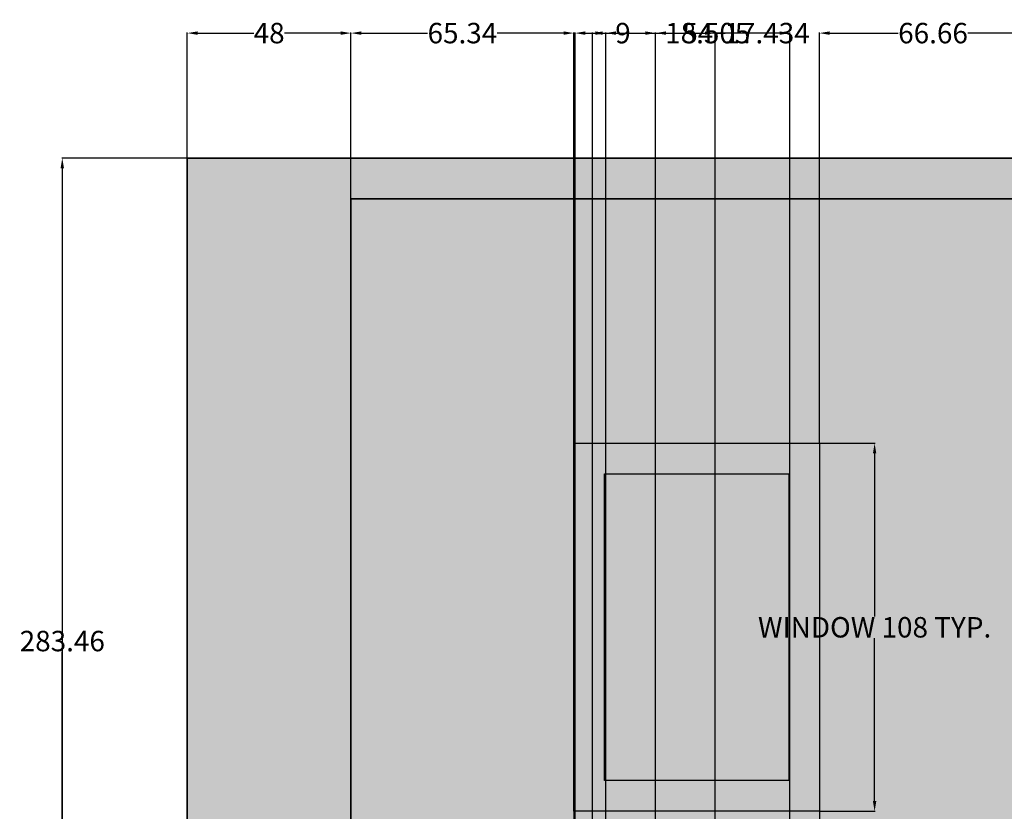
# Model space of a CAD drawing. Units: inches. Extents: x 126 to 726, y 86 to 888.
# Tile 8 of 13: x 137 to 426, y 655 to 888. Entities that reach past the tile are written whole.
import ezdxf

# ---------------------------------------------------------------- set-up
doc = ezdxf.new("R2010")
doc.units = ezdxf.units.IN
doc.header["$MEASUREMENT"] = 0
for name, color, linetype, lineweight in [('A-ANNO-DIMS', 2, 'Continuous', 18), ('A-ELEV', 7, 'Continuous', 35), ('A-ELEV-PATT', 8, 'Continuous', 13), ('A-GLAZ', 4, 'Continuous', 25)]:
    doc.layers.add(name, color=color, linetype=linetype, lineweight=lineweight)
doc.styles.get("Standard").update_dxf_attribs({"font": 'arial.ttf'})
doc.dimstyles.get("Standard").update_dxf_attribs({"dimtxt": 6, "dimasz": 3, "dimexe": 0.18, "dimexo": 0.0625, "dimgap": 0.09, "dimtad": 0, "dimtih": 1, "dimtoh": 1, "dimdec": 0, "dimzin": 0, "dimdsep": 46, "dimlunit": 3, "dimtxsty": 'Standard', "dimcen": 0.09, "dimadec": 0, "dimazin": 0, "dimtfac": 1, "dimtdec": 0, "dimtofl": 0, "dimtmove": 0, "dimatfit": 3, "dimfxl": 1, "dimtolj": 1, "dimtzin": 0, "dimarcsym": 0})

# ---------------------------------------------------------------- blocks, each defined once
blk = doc.blocks.new('WIN-FRAME')
for points in [[(72, 0), (0, 0), (0, 108), (72, 108)], [(63, 9), (9, 9), (9, 99), (63, 99)]]:
    blk.add_lwpolyline(points, close=True)
blk = doc.blocks.new('*D5')
at = {"layer": 'A-ANNO-DIMS', "color": 0, "lineweight": -2, "transparency": 16777216}
for p, q in [((371.38, 763.35), (387.7, 763.35)), ((387.52, 760.35), (387.52, 712.55)), ((387.52, 658.35), (387.52, 706.16)), ((371.38, 655.35), (387.7, 655.35))]:
    blk.add_line(p, q, dxfattribs=at)
at = {"layer": 'A-ANNO-DIMS', "color": 0, "transparency": 16777216}
for points in [[(387.02, 760.35), (388.02, 760.35), (387.52, 763.35)], [(387.02, 658.35), (388.02, 658.35), (387.52, 655.35)]]:
    blk.add_solid(points, dxfattribs=at)
at = {"layer": 'Defpoints', "color": 0, "transparency": 16777216}
for p in [(371.32, 763.35), (387.52, 763.35), (371.32, 655.35)]:
    blk.add_point(p, dxfattribs=at)
at = {"layer": 'A-ANNO-DIMS', "color": 0, "transparency": 16777216, "insert": (387.52, 709.35), "char_height": 6, "attachment_point": 5}
blk.add_mtext('\\A1;WINDOW 108 TYP.', dxfattribs=at)
blk = doc.blocks.new('*D6')
at = {"layer": 'A-ANNO-DIMS', "color": 0, "lineweight": -2, "transparency": 16777216}
for p, q in [((299.32, 655.29), (299.32, 638.97)), ((371.32, 655.29), (371.32, 638.97)), ((302.32, 639.15), (320.65, 639.15)), ((368.32, 639.15), (349.99, 639.15))]:
    blk.add_line(p, q, dxfattribs=at)
at = {"layer": 'A-ANNO-DIMS', "color": 0, "transparency": 16777216}
for points in [[(302.32, 639.65), (302.32, 638.65), (299.32, 639.15)], [(368.32, 639.65), (368.32, 638.65), (371.32, 639.15)]]:
    blk.add_solid(points, dxfattribs=at)
at = {"layer": 'Defpoints', "color": 0, "transparency": 16777216}
for p in [(299.32, 655.35), (371.32, 655.35), (371.32, 639.15)]:
    blk.add_point(p, dxfattribs=at)
at = {"layer": 'A-ANNO-DIMS', "color": 0, "transparency": 16777216, "insert": (335.32, 639.15), "char_height": 6, "attachment_point": 5}
blk.add_mtext('\\A1;72 TYP.', dxfattribs=at)
blk = doc.blocks.new('*D14')
at = {"layer": 'A-ANNO-DIMS', "color": 0, "lineweight": -2, "transparency": 16777216}
for p, q in [((185.91, 847.04), (149.14, 847.04)), ((149.32, 844.04), (149.32, 490.2)), ((149.32, 130.04), (149.32, 483.89)), ((185.91, 127.04), (149.14, 127.04))]:
    blk.add_line(p, q, dxfattribs=at)
at = {"layer": 'A-ANNO-DIMS', "color": 0, "transparency": 16777216}
for points in [[(148.82, 844.04), (149.82, 844.04), (149.32, 847.04)], [(148.82, 130.04), (149.82, 130.04), (149.32, 127.04)]]:
    blk.add_solid(points, dxfattribs=at)
at = {"layer": 'Defpoints', "color": 0, "transparency": 16777216}
for p in [(149.32, 847.04), (185.97, 847.04), (185.97, 127.04)]:
    blk.add_point(p, dxfattribs=at)
at = {"layer": 'A-ANNO-DIMS', "color": 0, "transparency": 16777216, "insert": (149.32, 487.04), "char_height": 6, "attachment_point": 5}
blk.add_mtext('\\A1;720', dxfattribs=at)
blk = doc.blocks.new('*D22')
at = {"layer": 'A-ANNO-DIMS', "color": 0, "lineweight": -2, "transparency": 16777216}
for p, q in [((185.91, 847.04), (149.14, 847.04)), ((149.32, 844.04), (149.32, 708.47)), ((149.32, 566.58), (149.32, 702.16)), ((431.28, 563.58), (149.14, 563.58))]:
    blk.add_line(p, q, dxfattribs=at)
at = {"layer": 'A-ANNO-DIMS', "color": 0, "transparency": 16777216}
for points in [[(148.82, 844.04), (149.82, 844.04), (149.32, 847.04)], [(148.82, 566.58), (149.82, 566.58), (149.32, 563.58)]]:
    blk.add_solid(points, dxfattribs=at)
at = {"layer": 'Defpoints', "color": 0, "transparency": 16777216}
for p in [(149.32, 847.04), (185.97, 847.04), (431.34, 563.58)]:
    blk.add_point(p, dxfattribs=at)
at = {"layer": 'A-ANNO-DIMS', "color": 0, "transparency": 16777216, "insert": (149.32, 705.31), "char_height": 6, "attachment_point": 5}
blk.add_mtext('\\A1;283.46', dxfattribs=at)
blk = doc.blocks.new('*D23')
at = {"layer": 'A-ANNO-DIMS', "color": 0, "lineweight": -2, "transparency": 16777216}
for p, q in [((185.97, 847.1), (185.97, 883.87)), ((188.97, 883.69), (205.46, 883.69)), ((230.97, 883.69), (214.49, 883.69)), ((233.97, 835.1), (233.97, 883.87))]:
    blk.add_line(p, q, dxfattribs=at)
at = {"layer": 'A-ANNO-DIMS', "color": 0, "transparency": 16777216}
for points in [[(188.97, 884.19), (188.97, 883.19), (185.97, 883.69)], [(230.97, 884.19), (230.97, 883.19), (233.97, 883.69)]]:
    blk.add_solid(points, dxfattribs=at)
at = {"layer": 'Defpoints', "color": 0, "transparency": 16777216}
for p in [(233.97, 883.69), (185.97, 847.04), (233.97, 835.04)]:
    blk.add_point(p, dxfattribs=at)
at = {"layer": 'A-ANNO-DIMS', "color": 0, "transparency": 16777216, "insert": (209.97, 883.69), "char_height": 6, "attachment_point": 5}
blk.add_mtext('\\A1;48', dxfattribs=at)
blk = doc.blocks.new('*D24')
at = {"layer": 'A-ANNO-DIMS', "color": 0, "lineweight": -2, "transparency": 16777216}
for p, q in [((233.97, 835.1), (233.97, 883.87)), ((236.97, 883.69), (256.43, 883.69)), ((296.32, 883.69), (276.86, 883.69)), ((299.32, 763.42), (299.32, 883.87))]:
    blk.add_line(p, q, dxfattribs=at)
at = {"layer": 'A-ANNO-DIMS', "color": 0, "transparency": 16777216}
for points in [[(236.97, 884.19), (236.97, 883.19), (233.97, 883.69)], [(296.32, 884.19), (296.32, 883.19), (299.32, 883.69)]]:
    blk.add_solid(points, dxfattribs=at)
at = {"layer": 'Defpoints', "color": 0, "transparency": 16777216}
for p in [(299.32, 883.69), (233.97, 835.04), (299.32, 763.35)]:
    blk.add_point(p, dxfattribs=at)
at = {"layer": 'A-ANNO-DIMS', "color": 0, "transparency": 16777216, "insert": (266.65, 883.69), "char_height": 6, "attachment_point": 5}
blk.add_mtext('\\A1;65.34', dxfattribs=at)
blk = doc.blocks.new('*D25')
at = {"layer": 'A-ANNO-DIMS', "color": 0, "lineweight": -2, "transparency": 16777216}
for p, q in [((371.32, 763.42), (371.32, 883.87)), ((374.32, 883.69), (394.42, 883.69)), ((434.97, 883.69), (414.87, 883.69)), ((437.97, 826.04), (437.97, 883.87))]:
    blk.add_line(p, q, dxfattribs=at)
at = {"layer": 'A-ANNO-DIMS', "color": 0, "transparency": 16777216}
for points in [[(374.32, 884.19), (374.32, 883.19), (371.32, 883.69)], [(434.97, 884.19), (434.97, 883.19), (437.97, 883.69)]]:
    blk.add_solid(points, dxfattribs=at)
at = {"layer": 'Defpoints', "color": 0, "transparency": 16777216}
for p in [(437.97, 883.69), (437.97, 825.98), (371.32, 763.35)]:
    blk.add_point(p, dxfattribs=at)
at = {"layer": 'A-ANNO-DIMS', "color": 0, "transparency": 16777216, "insert": (404.65, 883.69), "char_height": 6, "attachment_point": 5}
blk.add_mtext('\\A1;66.66', dxfattribs=at)
blk = doc.blocks.new('*D32')
at = {"layer": 'A-ANNO-DIMS', "color": 0, "lineweight": -2, "transparency": 16777216}
for p, q in [((299.67, 533.75), (299.67, 883.87)), ((302.67, 883.69), (305.67, 883.69)), ((308.67, 524.75), (308.67, 883.87)), ((308.67, 883.69), (311.67, 883.69))]:
    blk.add_line(p, q, dxfattribs=at)
at = {"layer": 'A-ANNO-DIMS', "color": 0, "transparency": 16777216}
for points in [[(302.67, 884.19), (302.67, 883.19), (299.67, 883.69)], [(305.67, 884.19), (305.67, 883.19), (308.67, 883.69)]]:
    blk.add_solid(points, dxfattribs=at)
at = {"layer": 'Defpoints', "color": 0, "transparency": 16777216}
for p in [(308.67, 883.69), (299.67, 533.68), (308.67, 524.68)]:
    blk.add_point(p, dxfattribs=at)
at = {"layer": 'A-ANNO-DIMS', "color": 0, "transparency": 16777216, "insert": (313.73, 883.69), "char_height": 6, "attachment_point": 5}
blk.add_mtext('\\A1;9', dxfattribs=at)
blk = doc.blocks.new('*D33')
at = {"layer": 'A-ANNO-DIMS', "color": 0, "lineweight": -2, "transparency": 16777216}
for p, q in [((308.67, 524.75), (308.67, 883.87)), ((311.67, 883.69), (331.29, 883.69)), ((359.67, 883.69), (340.04, 883.69)), ((362.67, 524.75), (362.67, 883.87))]:
    blk.add_line(p, q, dxfattribs=at)
at = {"layer": 'A-ANNO-DIMS', "color": 0, "transparency": 16777216}
for points in [[(311.67, 884.19), (311.67, 883.19), (308.67, 883.69)], [(359.67, 884.19), (359.67, 883.19), (362.67, 883.69)]]:
    blk.add_solid(points, dxfattribs=at)
at = {"layer": 'Defpoints', "color": 0, "transparency": 16777216}
for p in [(362.67, 883.69), (308.67, 524.68), (362.67, 524.68)]:
    blk.add_point(p, dxfattribs=at)
at = {"layer": 'A-ANNO-DIMS', "color": 0, "transparency": 16777216, "insert": (335.67, 883.69), "char_height": 6, "attachment_point": 5}
blk.add_mtext('\\A1;54', dxfattribs=at)
blk = doc.blocks.new('*D38')
at = {"layer": 'A-ANNO-DIMS', "color": 0, "lineweight": -2, "transparency": 16777216}
for p, q in [((304.8, 168.3), (304.8, 883.87)), ((307.8, 883.69), (320.3, 883.69)), ((323.3, 174.45), (323.3, 883.87)), ((323.3, 883.69), (326.3, 883.69))]:
    blk.add_line(p, q, dxfattribs=at)
at = {"layer": 'A-ANNO-DIMS', "color": 0, "transparency": 16777216}
for points in [[(307.8, 884.19), (307.8, 883.19), (304.8, 883.69)], [(320.3, 884.19), (320.3, 883.19), (323.3, 883.69)]]:
    blk.add_solid(points, dxfattribs=at)
at = {"layer": 'Defpoints', "color": 0, "transparency": 16777216}
for p in [(323.3, 883.69), (323.3, 174.39), (304.8, 168.24)]:
    blk.add_point(p, dxfattribs=at)
at = {"layer": 'A-ANNO-DIMS', "color": 0, "transparency": 16777216, "insert": (338.59, 883.69), "char_height": 6, "attachment_point": 5}
blk.add_mtext('\\A1;18.505', dxfattribs=at)
blk = doc.blocks.new('*D39')
at = {"layer": 'A-ANNO-DIMS', "color": 0, "lineweight": -2, "transparency": 16777216}
for p, q in [((323.3, 174.45), (323.3, 883.87)), ((326.3, 883.69), (337.74, 883.69)), ((340.74, 168.3), (340.74, 883.87)), ((340.74, 883.69), (343.74, 883.69))]:
    blk.add_line(p, q, dxfattribs=at)
at = {"layer": 'A-ANNO-DIMS', "color": 0, "transparency": 16777216}
for points in [[(326.3, 884.19), (326.3, 883.19), (323.3, 883.69)], [(337.74, 884.19), (337.74, 883.19), (340.74, 883.69)]]:
    blk.add_solid(points, dxfattribs=at)
at = {"layer": 'Defpoints', "color": 0, "transparency": 16777216}
for p in [(340.74, 883.69), (323.3, 174.39), (340.74, 168.24)]:
    blk.add_point(p, dxfattribs=at)
at = {"layer": 'A-ANNO-DIMS', "color": 0, "transparency": 16777216, "insert": (355.99, 883.69), "char_height": 6, "attachment_point": 5}
blk.add_mtext('\\A1;17.434', dxfattribs=at)

msp = doc.modelspace()

# ---------------------------------------------------------------- hatches: boundary and pattern name
at = {"layer": 'A-ELEV-PATT'}
h = msp.add_hatch(color=256, dxfattribs=at)
h.dxf.hatch_style = 1
h.paths.add_polyline_path([(233.9749, 545.5846), (431.3386, 545.5846), (431.3386, 563.5846), (185.9749, 563.5846), (185.9749, 395.5846), (431.3386, 395.5846), (431.3386, 413.5846), (233.9749, 413.5846)])
h.paths.add_polyline_path([(233.9749, 835.0424), (485.9749, 835.0424), (605.9749, 835.0424), (605.9749, 847.0424), (485.9749, 847.0424), (185.9749, 847.0424), (185.9749, 606.5846), (233.9749, 606.5846)])
h.paths.add_polyline_path([(233.9749, 597.5846), (185.9749, 597.5846), (185.9749, 585.5846), (233.9749, 585.5846)])
h.paths.add_polyline_path([(233.9749, 580.5846), (185.9749, 580.5846), (185.9749, 568.5846), (233.9749, 568.5846)])
h = msp.add_hatch(color=256, dxfattribs=at)
h.dxf.hatch_style = 1
h.paths.add_polyline_path([(437.9749, 499.1312), (485.9749, 499.1312), (485.9749, 501.4423), (437.9749, 501.4423), (437.9749, 513.4423), (485.9749, 513.4423), (485.9749, 515.7534), (437.9749, 515.7534), (437.9749, 527.7534), (485.9749, 527.7534), (485.9749, 530.0646), (437.9749, 530.0646), (437.9749, 542.0646), (485.9749, 542.0646), (485.9749, 544.3757), (437.9749, 544.3757), (437.9749, 556.3757), (485.9749, 556.3757), (485.9749, 558.6868), (437.9749, 558.6868), (437.9749, 570.6868), (485.9749, 570.6868), (485.9749, 572.9979), (437.9749, 572.9979), (437.9749, 584.9979), (485.9749, 584.9979), (485.9749, 587.309), (437.9749, 587.309), (437.9749, 595.0424), (429.9749, 595.0424), (429.9749, 607.0424), (437.9749, 607.0424), (437.9749, 615.9312), (437.9749, 630.2423), (437.9749, 642.2423), (485.9749, 642.2423), (485.9749, 644.5534), (437.9749, 644.5534), (437.9749, 656.5534), (485.9749, 656.5534), (485.9749, 658.8645), (437.9749, 658.8645), (437.9749, 670.8645), (485.9749, 670.8645), (485.9749, 673.1757), (437.9749, 673.1757), (437.9749, 685.1757), (485.9749, 685.1757), (485.9749, 687.4868), (437.9749, 687.4868), (437.9749, 699.4868), (485.9749, 699.4868), (485.9749, 701.7979), (437.9749, 701.7979), (437.9749, 713.7979), (485.9749, 713.7979), (485.9749, 716.109), (437.9749, 716.109), (437.9749, 728.109), (485.9749, 728.109), (485.9749, 730.4201), (437.9749, 730.4201), (437.9749, 742.4201), (485.9749, 742.4201), (485.9749, 744.7312), (437.9749, 744.7312), (437.9749, 756.7312), (485.9749, 756.7312), (485.9749, 759.0423), (437.9749, 759.0423), (437.9749, 771.0423), (485.9749, 771.0423), (485.9749, 773.3534), (437.9749, 773.3534), (437.9749, 785.3534), (485.9749, 785.3534), (485.9749, 787.6645), (437.9749, 787.6645), (437.9749, 799.6645), (485.9749, 799.6645), (485.9749, 801.9756), (437.9749, 801.9756), (437.9749, 811.2868), (485.9749, 811.2868), (485.9749, 813.9756), (437.9749, 813.9756), (437.9749, 825.9756), (485.9749, 825.9756), (485.9749, 835.0424), (233.9749, 835.0424), (233.9749, 606.5846), (185.9749, 606.5846), (185.9749, 597.5846), (233.9749, 597.5846), (233.9749, 585.5846), (185.9749, 585.5846), (185.9749, 580.5846), (233.9749, 580.5846), (233.9749, 568.5846), (185.9749, 568.5846), (185.9749, 563.5846), (431.3386, 563.5846), (431.3386, 545.5846), (233.9749, 545.5846), (233.9749, 413.5846), (431.3386, 413.5846), (431.3386, 395.5846), (185.9749, 395.5846), (185.9749, 386.5846), (233.9749, 386.5846), (233.9749, 374.5846), (185.9749, 374.5846), (185.9749, 369.5846), (233.9749, 369.5846), (233.9749, 357.5846), (185.9749, 357.5846), (185.9749, 352.5846), (233.9749, 352.5846), (233.9749, 340.5846), (185.9749, 340.5846), (185.9749, 331.5846), (233.9749, 331.5846), (233.9749, 127.0424), (485.9749, 127.0424), (485.9749, 129.3535), (437.9749, 129.3535), (437.9749, 141.3535), (485.9749, 141.3535), (485.9749, 143.6646), (437.9749, 143.6646), (437.9749, 155.6646), (485.9749, 155.6646), (485.9749, 157.9757), (437.9749, 157.9757), (437.9749, 169.9757), (485.9749, 169.9757), (485.9749, 172.2868), (437.9749, 172.2868), (437.9749, 184.2868), (485.9749, 184.2868), (485.9749, 186.5979), (437.9749, 186.5979), (437.9749, 198.5979), (485.9749, 198.5979), (485.9749, 200.909), (437.9749, 200.909), (437.9749, 212.909), (485.9749, 212.909), (485.9749, 215.2201), (437.9749, 215.2201), (437.9749, 227.2201), (485.9749, 227.2201), (485.9749, 229.5312), (437.9749, 229.5312), (437.9749, 241.5312), (485.9749, 241.5312), (485.9749, 243.8424), (437.9749, 243.8424), (437.9749, 255.8424), (485.9749, 255.8424), (485.9749, 258.1535), (437.9749, 258.1535), (437.9749, 270.1535), (485.9749, 270.1535), (485.9749, 272.4646), (437.9749, 272.4646), (437.9749, 284.4646), (485.9749, 284.4646), (485.9749, 286.7757), (437.9749, 286.7757), (437.9749, 298.7757), (485.9749, 298.7757), (485.9749, 301.0868), (437.9749, 301.0868), (437.9749, 313.0868), (485.9749, 313.0868), (485.9749, 315.3979), (437.9749, 315.3979), (437.9749, 327.3979), (485.9749, 327.3979), (485.9749, 329.709), (437.9749, 329.709), (437.9749, 341.709), (485.9749, 341.709), (485.9749, 344.0201), (437.9749, 344.0201), (437.9749, 355.0424), (429.9749, 355.0424), (429.9749, 367.0424), (437.9749, 367.0424), (437.9749, 372.6423), (437.9749, 386.9535), (437.9749, 401.2646), (437.9749, 413.2646), (485.9749, 413.2646), (485.9749, 415.5757), (437.9749, 415.5757), (437.9749, 427.5757), (485.9749, 427.5757), (485.9749, 429.8868), (437.9749, 429.8868), (437.9749, 441.8868), (485.9749, 441.8868), (485.9749, 444.1979), (437.9749, 444.1979), (437.9749, 456.1979), (485.9749, 456.1979), (485.9749, 458.509), (437.9749, 458.509), (437.9749, 470.509), (485.9749, 470.509), (485.9749, 472.8201), (437.9749, 472.8201), (437.9749, 484.8201), (485.9749, 484.8201), (485.9749, 487.1312), (437.9749, 487.1312)])
h.paths.add_polyline_path([(299.6658, 533.6845), (371.6658, 533.6845), (371.6658, 425.6845), (299.6658, 425.6845)], flags=16)
h.paths.add_polyline_path([(308.6658, 524.6845), (362.6658, 524.6845), (362.6658, 434.6845), (308.6658, 434.6845)], flags=0)
h.paths.add_polyline_path([(317.7956, 603.3211, -0.4129833), (306.8418, 614.321, -0.94403766), (328.769, 615.5845, -0.04423165), (330.7031, 615.4048, -0.89973713), (352.5798, 615.6161, -0.4129833), (363.5336, 604.6162, -0.94403766), (341.6064, 603.3528, -0.04423165), (339.6723, 603.5324, -0.89973713)], flags=16)
h.paths.add_polyline_path([(319.7228, 604.5846, -0.02633223), (319.7726, 605.5306, -0.47905713), (308.8418, 614.321, -1), (326.8418, 614.321, -0.02633223), (326.7919, 613.375, -0.17413188), (332.826, 612.5948, -0.04918553), (332.6526, 614.3527, -1), (350.6526, 614.3527, -0.02633223), (350.6028, 613.4067, -0.47905713), (361.5336, 604.6162, -1), (343.5336, 604.6162, -0.02633223), (343.5834, 605.5622, -0.17413188), (337.5494, 606.3424, -0.04918553), (337.7228, 604.5846, -1)], flags=0)
h.paths.add_polyline_path([(328.769, 355.6561, -0.04423165), (330.7031, 355.4765, -0.89973713), (352.5798, 355.6878, -0.4129833), (363.5336, 344.6879, -0.94403766), (341.6064, 343.4244, -0.04423165), (339.6723, 343.604, -0.89973713), (317.7956, 343.3927, -0.4129833), (306.8418, 354.3926, -0.94403766)], flags=16)
h.paths.add_polyline_path([(326.8418, 354.3926, -0.02633223), (326.7919, 353.4466, -0.17413188), (332.826, 352.6664, -0.04918553), (332.6526, 354.4243, -1), (350.6526, 354.4243, -0.02633223), (350.6028, 353.4783, -0.47905713), (361.5336, 344.6879, -1), (343.5336, 344.6879, -0.02633223), (343.5834, 345.6339, -0.17413188), (337.5494, 346.4141, -0.04918553), (337.7228, 344.6562, -1), (319.7228, 344.6562, -0.02633223), (319.7726, 345.6022, -0.47905713), (308.8418, 354.3926, -1)], flags=0)
h.paths.add_polyline_path([(299.3189, 655.3527), (299.3189, 763.3527), (371.3189, 763.3527), (371.3189, 655.3527)], flags=16)
h.paths.add_polyline_path([(308.3189, 664.3527), (308.3189, 754.3527), (362.3189, 754.3527), (362.3189, 664.3527)], flags=0)
h.paths.add_polyline_path([(299.6658, 303.5875), (371.6658, 303.5875), (371.6658, 195.5875), (299.6658, 195.5875)], flags=16)
h.paths.add_polyline_path([(308.6658, 294.5875), (362.6658, 294.5875), (362.6658, 204.5875), (308.6658, 204.5875)], flags=0)
h.paths.add_polyline_path([(326.3038, 177.3867), (346.055, 177.3867, -0.41421356), (349.055, 174.3867), (349.055, 171.2378), (363.489, 171.2378, -0.41421356), (366.489, 168.2378), (366.489, 159.7133, -0.41421356), (363.489, 156.7133), (343.7379, 156.7133, -0.41421356), (340.7379, 159.7133), (340.7379, 162.8622), (330.5504, 162.8622), (330.5504, 159.7133, -0.41421356), (327.5504, 156.7133), (307.7992, 156.7133, -0.41421356), (304.7992, 159.7133), (304.7992, 168.2378, -0.41421356), (307.7992, 171.2378), (323.3038, 171.2378), (323.3038, 174.3867, -0.41421356)], flags=16)
h.paths.add_polyline_path([(326.3038, 175.3867), (346.055, 175.3867, -0.41421356), (347.055, 174.3867), (347.055, 169.2378), (363.489, 169.2378, -0.41421356), (364.489, 168.2378), (364.489, 159.7133, -0.41421356), (363.489, 158.7133), (343.7379, 158.7133, -0.41421356), (342.7379, 159.7133), (342.7379, 164.8622), (328.5504, 164.8622), (328.5504, 159.7133, -0.41421356), (327.5504, 158.7133), (307.7992, 158.7133, -0.41421356), (306.7992, 159.7133), (306.7992, 168.2378, -0.41421356), (307.7992, 169.2378), (325.3038, 169.2378), (325.3038, 174.3867, -0.41421356)], flags=0)
h = msp.add_hatch(dxfattribs=at)
h.set_pattern_fill('GRAVEL', color=256, scale=40)
h.paths.add_polyline_path([(437.9749, 642.2423), (485.9749, 642.2423), (485.9749, 644.5534), (437.9749, 644.5534), (437.9749, 656.5534), (485.9749, 656.5534), (485.9749, 658.8645), (437.9749, 658.8645), (437.9749, 670.8645), (485.9749, 670.8645), (485.9749, 673.1757), (437.9749, 673.1757), (437.9749, 685.1757), (485.9749, 685.1757), (485.9749, 687.4868), (437.9749, 687.4868), (437.9749, 699.4868), (485.9749, 699.4868), (485.9749, 701.7979), (437.9749, 701.7979), (437.9749, 713.7979), (485.9749, 713.7979), (485.9749, 716.109), (437.9749, 716.109), (437.9749, 728.109), (485.9749, 728.109), (485.9749, 730.4201), (437.9749, 730.4201), (437.9749, 742.4201), (485.9749, 742.4201), (485.9749, 744.7312), (437.9749, 744.7312), (437.9749, 756.7312), (485.9749, 756.7312), (485.9749, 759.0423), (437.9749, 759.0423), (437.9749, 771.0423), (485.9749, 771.0423), (485.9749, 773.3534), (437.9749, 773.3534), (437.9749, 785.3534), (485.9749, 785.3534), (485.9749, 787.6645), (437.9749, 787.6645), (437.9749, 799.6645), (485.9749, 799.6645), (485.9749, 801.9756), (437.9749, 801.9756), (437.9749, 811.2868), (485.9749, 811.2868), (485.9749, 813.9756), (437.9749, 813.9756), (437.9749, 825.9756), (485.9749, 825.9756), (485.9749, 835.0424), (233.9749, 835.0424), (233.9749, 606.5846), (185.9749, 606.5846), (185.9749, 597.5846), (233.9749, 597.5846), (233.9749, 585.5846), (185.9749, 585.5846), (185.9749, 580.5846), (233.9749, 580.5846), (233.9749, 568.5846), (185.9749, 568.5846), (185.9749, 563.5846), (431.3386, 563.5846), (431.3386, 545.5846), (233.9749, 545.5846), (233.9749, 413.5846), (431.3386, 413.5846), (431.3386, 395.5846), (185.9749, 395.5846), (185.9749, 386.5846), (233.9749, 386.5846), (233.9749, 374.5846), (185.9749, 374.5846), (185.9749, 369.5846), (233.9749, 369.5846), (233.9749, 357.5846), (185.9749, 357.5846), (185.9749, 352.5846), (233.9749, 352.5846), (233.9749, 340.5846), (185.9749, 340.5846), (185.9749, 331.5846), (233.9749, 331.5846), (233.9749, 127.0424), (485.9749, 127.0424), (485.9749, 129.3535), (437.9749, 129.3535), (437.9749, 141.3535), (485.9749, 141.3535), (485.9749, 143.6646), (437.9749, 143.6646), (437.9749, 155.6646), (485.9749, 155.6646), (485.9749, 157.9757), (437.9749, 157.9757), (437.9749, 169.9757), (485.9749, 169.9757), (485.9749, 172.2868), (437.9749, 172.2868), (437.9749, 184.2868), (485.9749, 184.2868), (485.9749, 186.5979), (437.9749, 186.5979), (437.9749, 198.5979), (485.9749, 198.5979), (485.9749, 200.909), (437.9749, 200.909), (437.9749, 212.909), (485.9749, 212.909), (485.9749, 215.2201), (437.9749, 215.2201), (437.9749, 227.2201), (485.9749, 227.2201), (485.9749, 229.5312), (437.9749, 229.5312), (437.9749, 241.5312), (485.9749, 241.5312), (485.9749, 243.8424), (437.9749, 243.8424), (437.9749, 255.8424), (485.9749, 255.8424), (485.9749, 258.1535), (437.9749, 258.1535), (437.9749, 270.1535), (485.9749, 270.1535), (485.9749, 272.4646), (437.9749, 272.4646), (437.9749, 284.4646), (485.9749, 284.4646), (485.9749, 286.7757), (437.9749, 286.7757), (437.9749, 298.7757), (485.9749, 298.7757), (485.9749, 301.0868), (437.9749, 301.0868), (437.9749, 313.0868), (485.9749, 313.0868), (485.9749, 315.3979), (437.9749, 315.3979), (437.9749, 327.3979), (485.9749, 327.3979), (485.9749, 329.709), (437.9749, 329.709), (437.9749, 341.709), (485.9749, 341.709), (485.9749, 344.0201), (437.9749, 344.0201), (437.9749, 355.0424), (429.9749, 355.0424), (429.9749, 367.0424), (437.9749, 367.0424), (437.9749, 372.6423), (437.9749, 386.9535), (437.9749, 401.2646), (437.9749, 413.2646), (485.9749, 413.2646), (485.9749, 415.5757), (437.9749, 415.5757), (437.9749, 427.5757), (485.9749, 427.5757), (485.9749, 429.8868), (437.9749, 429.8868), (437.9749, 441.8868), (485.9749, 441.8868), (485.9749, 444.1979), (437.9749, 444.1979), (437.9749, 456.1979), (485.9749, 456.1979), (485.9749, 458.509), (437.9749, 458.509), (437.9749, 470.509), (485.9749, 470.509), (485.9749, 472.8201), (437.9749, 472.8201), (437.9749, 484.8201), (485.9749, 484.8201), (485.9749, 487.1312), (437.9749, 487.1312), (437.9749, 499.1312), (485.9749, 499.1312), (485.9749, 501.4423), (437.9749, 501.4423), (437.9749, 513.4423), (485.9749, 513.4423), (485.9749, 515.7534), (437.9749, 515.7534), (437.9749, 527.7534), (485.9749, 527.7534), (485.9749, 530.0646), (437.9749, 530.0646), (437.9749, 542.0646), (485.9749, 542.0646), (485.9749, 544.3757), (437.9749, 544.3757), (437.9749, 556.3757), (485.9749, 556.3757), (485.9749, 558.6868), (437.9749, 558.6868), (437.9749, 570.6868), (485.9749, 570.6868), (485.9749, 572.9979), (437.9749, 572.9979), (437.9749, 584.9979), (485.9749, 584.9979), (485.9749, 587.309), (437.9749, 587.309), (437.9749, 595.0424), (429.9749, 595.0424), (429.9749, 607.0424), (437.9749, 607.0424), (437.9749, 615.9312), (437.9749, 630.2423)])
h.paths.add_polyline_path([(371.3189, 655.3527), (299.3189, 655.3527), (299.3189, 763.3527), (371.3189, 763.3527)], flags=16)
h.paths.add_polyline_path([(363.5336, 604.6162, -0.94403766), (341.6064, 603.3528, -0.04423165), (339.6723, 603.5324, -0.89973713), (317.7956, 603.3211, -0.4129833), (306.8418, 614.321, -0.94403766), (328.769, 615.5845, -0.04423165), (330.7031, 615.4048, -0.89973713), (352.5798, 615.6161, -0.4129833)], flags=16)
h.paths.add_polyline_path([(361.5336, 604.6162, -1), (343.5336, 604.6162, -0.02633223), (343.5834, 605.5622, -0.17413188), (337.5494, 606.3424, -0.04918553), (337.7228, 604.5846, -1), (319.7228, 604.5846, -0.02633223), (319.7726, 605.5306, -0.47905713), (308.8418, 614.321, -1), (326.8418, 614.321, -0.02633223), (326.7919, 613.375, -0.17413188), (332.826, 612.5948, -0.04918553), (332.6526, 614.3527, -1), (350.6526, 614.3527, -0.02633223), (350.6028, 613.4067, -0.47905713)], flags=0)
h.paths.add_polyline_path([(362.3189, 664.3527), (308.3189, 664.3527), (308.3189, 754.3527), (362.3189, 754.3527)], flags=0)
h.paths.add_polyline_path([(371.6658, 533.6845), (371.6658, 425.6845), (299.6658, 425.6845), (299.6658, 533.6845)], flags=16)
h.paths.add_polyline_path([(362.6658, 524.6845), (362.6658, 434.6845), (308.6658, 434.6845), (308.6658, 524.6845)], flags=0)
h.paths.add_polyline_path([(352.5798, 355.6878, -0.4129833), (363.5336, 344.6879, -0.94403766), (341.6064, 343.4244, -0.04423165), (339.6723, 343.604, -0.89973713), (317.7956, 343.3927, -0.4129833), (306.8418, 354.3926, -0.94403766), (328.769, 355.6561, -0.04423165), (330.7031, 355.4765, -0.89973713)], flags=16)
h.paths.add_polyline_path([(350.6526, 354.4243, -0.02633223), (350.6028, 353.4783, -0.47905713), (361.5336, 344.6879, -1), (343.5336, 344.6879, -0.02633223), (343.5834, 345.6339, -0.17413188), (337.5494, 346.4141, -0.04918553), (337.7228, 344.6562, -1), (319.7228, 344.6562, -0.02633223), (319.7726, 345.6022, -0.47905713), (308.8418, 354.3926, -1), (326.8418, 354.3926, -0.02633223), (326.7919, 353.4466, -0.17413188), (332.826, 352.6664, -0.04918553), (332.6526, 354.4243, -1)], flags=0)
h.paths.add_polyline_path([(371.6658, 303.5875), (371.6658, 195.5875), (299.6658, 195.5875), (299.6658, 303.5875)], flags=16)
h.paths.add_polyline_path([(362.6658, 294.5875), (362.6658, 204.5875), (308.6658, 204.5875), (308.6658, 294.5875)], flags=0)
h.paths.add_polyline_path([(346.055, 177.3867, -0.41421356), (349.055, 174.3867), (349.055, 171.2378), (363.489, 171.2378, -0.41421356), (366.489, 168.2378), (366.489, 159.7133, -0.41421356), (363.489, 156.7133), (343.7379, 156.7133, -0.41421356), (340.7379, 159.7133), (340.7379, 162.8622), (330.5504, 162.8622), (330.5504, 159.7133, -0.41421356), (327.5504, 156.7133), (307.7992, 156.7133, -0.41421356), (304.7992, 159.7133), (304.7992, 168.2378, -0.41421356), (307.7992, 171.2378), (323.3038, 171.2378), (323.3038, 174.3867, -0.41421356), (326.3038, 177.3867)], flags=16)
h.paths.add_polyline_path([(346.055, 175.3867, -0.41421356), (347.055, 174.3867), (347.055, 169.2378), (363.489, 169.2378, -0.41421356), (364.489, 168.2378), (364.489, 159.7133, -0.41421356), (363.489, 158.7133), (343.7379, 158.7133, -0.41421356), (342.7379, 159.7133), (342.7379, 164.8622), (328.5504, 164.8622), (328.5504, 159.7133, -0.41421356), (327.5504, 158.7133), (307.7992, 158.7133, -0.41421356), (306.7992, 159.7133), (306.7992, 168.2378, -0.41421356), (307.7992, 169.2378), (325.3038, 169.2378), (325.3038, 174.3867, -0.41421356), (326.3038, 175.3867)], flags=0)
h = msp.add_hatch(color=256, dxfattribs=at)
h.dxf.hatch_style = 1
h.paths.add_polyline_path([(371.6658, 533.6845), (299.6658, 533.6845), (299.6658, 425.6845), (371.6658, 425.6845)])
h.paths.add_polyline_path([(362.6658, 434.6845), (308.6658, 434.6845), (308.6658, 524.6845), (362.6658, 524.6845)], flags=16)
h.paths.add_polyline_path([(371.3189, 763.3527), (299.3189, 763.3527), (299.3189, 655.3527), (371.3189, 655.3527)])
h.paths.add_polyline_path([(362.3189, 664.3527), (308.3189, 664.3527), (308.3189, 754.3527), (362.3189, 754.3527)], flags=16)
at = {"layer": 'A-GLAZ'}
h = msp.add_hatch(color=256, dxfattribs=at)
h.dxf.hatch_style = 1
h.paths.add_polyline_path([(362.3189, 754.3527), (308.3189, 754.3527), (308.3189, 664.3527), (362.3189, 664.3527)])

# ---------------------------------------------------------------- linework, layer by layer
at = {"layer": 'A-ELEV'}
for p, q in [((485.9749, 847.0424), (185.9749, 847.0424)), ((185.9749, 847.0424), (185.9749, 127.0424)), ((233.9749, 835.0424), (233.9749, 606.5846)), ((485.9749, 835.0424), (233.9749, 835.0424))]:
    msp.add_line(p, q, dxfattribs=at)

# ---------------------------------------------------------------- block references
at = {"layer": 'A-GLAZ'}
msp.add_blockref('WIN-FRAME', (299.319, 655.353), dxfattribs=at)

# ---------------------------------------------------------------- dimensions: what is measured, and where the dimension line sits
at = {"layer": 'A-ANNO-DIMS'}
for base, p1, p2, override, picture, middle in [((233.9749, 883.6924), (185.9749, 847.0424), (233.9749, 835.0424), {"dimdec": 0, "dimlfac": 1, "dimrnd": 0, "dimzin": 0, "dimdsep": 46, "dimlunit": 2}, '*D23', (209.9749, 883.6924)), ((299.3189, 883.6924), (233.9749, 835.0424), (299.3189, 763.3527), {"dimdec": 2, "dimlfac": 1, "dimrnd": 0, "dimzin": 0, "dimdsep": 46, "dimlunit": 2}, '*D24', (266.6469, 883.6924)), ((308.6658, 883.6924), (299.6658, 533.6845), (308.6658, 524.6845), {"dimdec": 0, "dimlfac": 1, "dimrnd": 0, "dimzin": 0, "dimdsep": 46, "dimlunit": 2}, '*D32', (313.7286, 883.6924)), ((323.3038, 883.6924), (304.7992, 168.2378), (323.3038, 174.3867), {"dimdec": 3, "dimlfac": 1, "dimrnd": 0, "dimzin": 0, "dimdsep": 46, "dimlunit": 2}, '*D38', (338.5882, 883.6924)), ((362.6658, 883.6924), (308.6658, 524.6845), (362.6658, 524.6845), {"dimdec": 0, "dimlfac": 1, "dimrnd": 0, "dimzin": 0, "dimdsep": 46, "dimlunit": 2}, '*D33', (335.6658, 883.6924)), ((340.7379, 883.6924), (323.3038, 174.3867), (340.7379, 168.2378), {"dimdec": 3, "dimlfac": 1, "dimrnd": 0, "dimzin": 0, "dimdsep": 46, "dimlunit": 2}, '*D39', (355.9875, 883.6924)), ((437.9749, 883.6924), (371.3189, 763.3527), (437.9749, 825.9756), {"dimdec": 2, "dimlfac": 1, "dimrnd": 0, "dimzin": 0, "dimdsep": 46, "dimlunit": 2}, '*D25', (404.6469, 883.6924))]:
    dim = msp.add_linear_dim(base=base, p1=p1, p2=p2, dimstyle='Standard', override=override, dxfattribs=at)
    dim.commit()
    dim.dimension.update_dxf_attribs({"geometry": picture, "text_midpoint": middle})
for p1, override, picture, middle in [((431.3386, 563.5846), {"dimdec": 2, "dimlfac": 1, "dimrnd": 0, "dimzin": 0, "dimdsep": 46, "dimlunit": 2}, '*D22', (149.3249, 705.3135)), ((185.9749, 127.0424), {"dimdec": 0, "dimlfac": 1, "dimrnd": 0, "dimzin": 0, "dimdsep": 46, "dimlunit": 2}, '*D14', (149.3249, 487.0424))]:
    dim = msp.add_linear_dim(base=(149.3249, 847.0424), p1=p1, p2=(185.9749, 847.0424), angle=90, dimstyle='Standard', override=override, dxfattribs=at)
    dim.commit()
    dim.dimension.update_dxf_attribs({"geometry": picture, "text_midpoint": middle})
dim = msp.add_linear_dim(base=(387.5189, 763.3527), p1=(371.3189, 655.3527), p2=(371.3189, 763.3527), angle=90, text='WINDOW <> TYP.', dimstyle='Standard', override={"dimdec": 0, "dimlfac": 1, "dimrnd": 0, "dimzin": 0, "dimdsep": 46, "dimlunit": 2}, dxfattribs=at)
dim.commit()
dim.dimension.update_dxf_attribs({"geometry": '*D5', "text_midpoint": (387.5189, 709.3527)})
dim = msp.add_linear_dim(base=(371.3189, 639.1527), p1=(299.3189, 655.3527), p2=(371.3189, 655.3527), text='<> TYP.', dimstyle='Standard', override={"dimdec": 0, "dimlfac": 1, "dimrnd": 0, "dimzin": 0, "dimdsep": 46, "dimlunit": 2}, dxfattribs=at)
dim.commit()
dim.dimension.update_dxf_attribs({"geometry": '*D6', "text_midpoint": (335.3189, 639.1527)})

doc.saveas('drawing.dxf')
